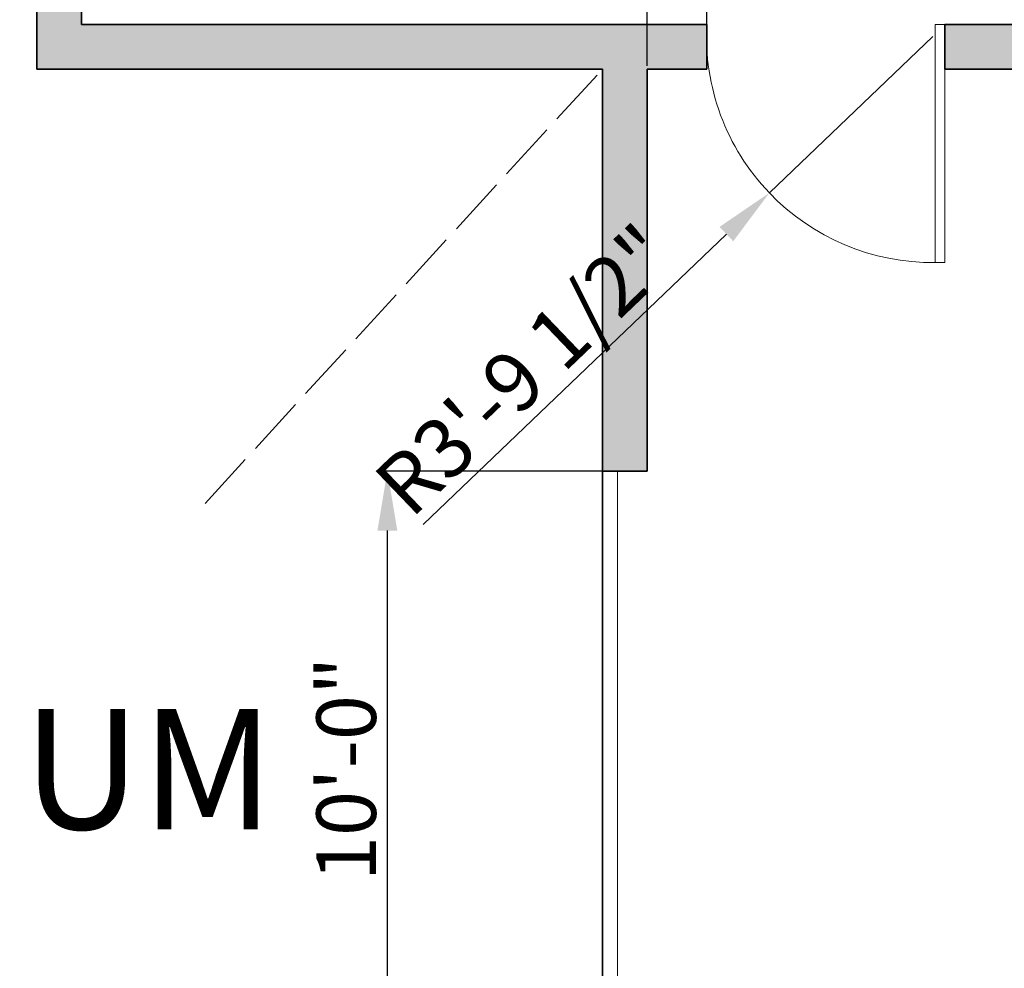
# Model space of a CAD drawing. Units: inches. Extents: x 2083 to 3317, y 1141 to 2115.
# Tile 116 of 256: x 2746 to 2944, y 1522 to 1713. Entities that reach past the tile are written whole.
import ezdxf

# ---------------------------------------------------------------- set-up
doc = ezdxf.new("R2010")
doc.units = ezdxf.units.IN
doc.linetypes.add('ACAD_ISO02W100', pattern=[15, 12, -3])
for name, color, linetype, lineweight in [('A-ANNO-DIMS', 2, 'Continuous', 18), ('A-AREA-IDEN', 7, 'Continuous', 25), ('A-DOOR', 4, 'Continuous', 18), ('A-FLOR-OPEN', 8, 'ACAD_ISO02W100', 13), ('A-GLAZ', 4, 'Continuous', 18), ('A-WALL', 7, 'Continuous', 35)]:
    doc.layers.add(name, color=color, linetype=linetype, lineweight=lineweight)
doc.layers.add('A-WALL-PATT', color=251, linetype='Continuous', lineweight=13, true_color=0x636466)
doc.styles.get("Standard").update_dxf_attribs({"font": 'arial.ttf'})
doc.dimstyles.new('ISO-25', dxfattribs={"dimtxt": 12, "dimasz": 12, "dimexe": 1.25, "dimexo": 0.625, "dimtad": 1, "dimlunit": 3, "dimtxsty": 'Standard', "dimcen": 2.5, "dimadec": 0, "dimazin": 0, "dimtfac": 1, "dimtmove": 0, "dimatfit": 3, "dimfxl": 1, "dimarcsym": 0})

# ---------------------------------------------------------------- blocks, each defined once
blk = doc.blocks.new('*D57')
at = {"layer": 'A-ANNO-DIMS', "color": 0, "lineweight": -2, "transparency": 16777216}
for p, q in [((2871.33, 1621.76), (2818.36, 1621.76)), ((2819.61, 1513.76), (2819.61, 1609.76)), ((2871.33, 1501.76), (2818.36, 1501.76))]:
    blk.add_line(p, q, dxfattribs=at)
at = {"layer": 'A-ANNO-DIMS', "color": 0, "transparency": 16777216}
for points in [[(2817.61, 1609.76), (2821.61, 1609.76), (2819.61, 1621.76)], [(2817.61, 1513.76), (2821.61, 1513.76), (2819.61, 1501.76)]]:
    blk.add_solid(points, dxfattribs=at)
at = {"layer": 'Defpoints', "color": 0, "transparency": 16777216}
for p in [(2819.61, 1621.76), (2871.96, 1621.76), (2871.96, 1501.76)]:
    blk.add_point(p, dxfattribs=at)
at = {"layer": 'A-ANNO-DIMS', "color": 0, "transparency": 16777216, "insert": (2812.86, 1561.76), "char_height": 12, "attachment_point": 5, "rotation": 90}
blk.add_mtext('10\'-0"', dxfattribs=at)
blk = doc.blocks.new('*D58')
at = {"layer": 'A-ANNO-DIMS', "color": 0, "lineweight": -2, "transparency": 16777216}
for p, q in [((2871.96, 1703.39), (2871.96, 1756.36)), ((2883.96, 1703.39), (2883.96, 1756.36)), ((2859.96, 1755.11), (2847.96, 1755.11)), ((2871.96, 1755.11), (2883.96, 1755.11)), ((2895.96, 1755.11), (2939.98, 1755.11))]:
    blk.add_line(p, q, dxfattribs=at)
at = {"layer": 'A-ANNO-DIMS', "color": 0, "transparency": 16777216}
for points in [[(2859.96, 1757.11), (2859.96, 1753.11), (2871.96, 1755.11)], [(2895.96, 1757.11), (2895.96, 1753.11), (2883.96, 1755.11)]]:
    blk.add_solid(points, dxfattribs=at)
at = {"layer": 'Defpoints', "color": 0, "transparency": 16777216}
for p in [(2883.96, 1755.11), (2871.96, 1702.76), (2883.96, 1702.76)]:
    blk.add_point(p, dxfattribs=at)
at = {"layer": 'A-ANNO-DIMS', "color": 0, "transparency": 16777216, "insert": (2923.97, 1761.86), "char_height": 12, "attachment_point": 5}
blk.add_mtext('1\'-0"', dxfattribs=at)
blk = doc.blocks.new('*D72')
at = {"layer": 'A-ANNO-DIMS', "color": 0, "lineweight": -2, "transparency": 16777216}
for p, q in [((2929.49, 1709.35), (2896.57, 1677.81)), ((2826.83, 1610.97), (2887.91, 1669.5))]:
    blk.add_line(p, q, dxfattribs=at)
at = {"layer": 'A-ANNO-DIMS', "color": 0, "transparency": 16777216}
blk.add_solid([(2886.52, 1670.95), (2889.29, 1668.06), (2896.57, 1677.81)], dxfattribs=at)
at = {"layer": 'Defpoints', "color": 0, "transparency": 16777216}
for p in [(2929.49, 1709.35), (2896.57, 1677.81)]:
    blk.add_point(p, dxfattribs=at)
at = {"layer": 'A-ANNO-DIMS', "color": 0, "transparency": 16777216, "insert": (2848.31, 1641.02), "char_height": 12, "attachment_point": 5, "rotation": 43.7815}
blk.add_mtext('R3\'-9 1/2"', dxfattribs=at)

msp = doc.modelspace()

# ---------------------------------------------------------------- hatches: boundary and pattern name
at = {"layer": 'A-WALL-PATT'}
h = msp.add_hatch(color=256, dxfattribs=at)
h.dxf.hatch_style = 1
h.paths.add_polyline_path([(3126.96, 2020.761), (2748.96, 2020.761), (2604.96, 2020.761), (2226.96, 2020.761), (2226.96, 1702.761), (2466.96, 1702.761), (2466.96, 1582.761), (2418.96, 1582.761), (2418.96, 1477.761), (2226.96, 1477.761), (2226.96, 1263.261), (2544.96, 1263.261), (2544.96, 1411.761), (2604.96, 1411.761), (2685.96, 1411.761), (2685.96, 1420.761), (2604.96, 1420.761), (2604.96, 1573.761), (2604.96, 1702.761), (2604.96, 2011.761), (2748.96, 2011.761), (2748.96, 1702.761), (2862.96, 1702.761), (2862.96, 1621.761), (2871.96, 1621.761), (2871.96, 1702.761), (2883.96, 1702.761), (2883.96, 1706.939, -0.0264593), (2883.96, 1711.761), (2757.96, 1711.761), (2757.96, 1807.761), (2787.96, 1807.761), (2787.96, 1812.261), (2757.96, 1812.261), (2757.96, 2011.761), (2877.96, 2011.761), (2877.96, 1812.261), (2847.96, 1812.261), (2847.96, 1807.761), (2889.836, 1807.761), (2889.836, 1812.261), (2882.46, 1812.261), (2882.46, 2011.761), (3117.96, 2011.761), (3117.96, 1812.261), (2937.836, 1812.261), (2937.836, 1807.761), (2995.71, 1807.761), (2995.71, 1796.118), (3000.21, 1796.118), (3000.21, 1807.761), (3117.96, 1807.761), (3117.96, 1711.761), (3000.21, 1711.761), (3000.21, 1760.118), (2998.573, 1760.118, -0.020711), (2995.71, 1760.118), (2995.71, 1711.761), (2931.96, 1711.761), (2931.96, 1702.761), (3126.96, 1702.761)])
h.paths.add_polyline_path([(2471.46, 2011.761), (2471.46, 1810.011), (2462.717, 1810.011), (2462.717, 1805.511), (2505.96, 1805.511), (2505.96, 1810.011), (2475.96, 1810.011), (2475.96, 2011.761), (2595.96, 2011.761), (2595.96, 1810.011), (2565.96, 1810.011), (2565.96, 1805.511), (2595.96, 1805.511), (2595.96, 1711.761), (2235.96, 1711.761), (2235.96, 1805.511), (2353.71, 1805.511), (2353.71, 1796.054), (2358.21, 1796.054), (2358.21, 1805.511), (2414.717, 1805.511), (2414.717, 1810.011), (2235.96, 1810.011), (2235.96, 2011.761)], flags=16)
h.paths.add_polyline_path([(2270.205, 1994.61), (2270.205, 1970.61), (2246.205, 1970.61), (2246.205, 1994.61)], flags=0)
edge = h.paths.add_edge_path(flags=0)
edge.add_ellipse((2332.027, 1899.798), major_axis=(-3.043, 3.043), ratio=0.1682525, start_angle=-161.33217, end_angle=-156.30711, ccw=False)
edge.add_ellipse((2333.082, 1898.744), major_axis=(-1.055, 1.055), ratio=0.4535321, start_angle=-123.37102, end_angle=-94.15911)
edge = h.paths.add_edge_path(flags=0)
edge.add_ellipse((2332.027, 1968.876), major_axis=(3.043, 3.043), ratio=0.1682525, start_angle=18.66783, end_angle=23.69289)
edge.add_spline(control_points=[(2332.926, 1970.691), (2332.227, 1970.336), (2330.894, 1969.659), (2328.413, 1970.932), (2327.204, 1967.749), (2324.71, 1969.956), (2322.533, 1967.012), (2320.013, 1971.296), (2317.68, 1968.158), (2316.041, 1967.102), (2315.427, 1966.81)], knot_values=[0, 0, 0, 0, 2.2670587, 4.3245589, 6.6855835, 8.8786411, 11.121502, 14.300359, 17.7552837, 19.732645, 19.732645, 19.732645, 19.732645], degree=3, periodic=0)
edge.add_ellipse((2332.027, 1968.876), major_axis=(3.043, 3.043), ratio=0.1682525, start_angle=18.66783, end_angle=23.69289, ccw=False)
edge.add_ellipse((2333.082, 1969.931), major_axis=(1.055, 1.055), ratio=0.4535321, start_angle=56.62898, end_angle=85.84089, ccw=False)
edge = h.paths.add_edge_path(flags=0)
edge.add_spline(control_points=[(2296.428, 1967.988), (2293.628, 1965.336), (2287.704, 1959.727), (2299.744, 1949.996), (2294.533, 1935.669), (2290.573, 1920.604), (2293.394, 1909.974), (2296.185, 1904.967)], knot_values=[0.0991853, 0.0991853, 0.0991853, 0.0991853, 0.3453009, 0.6198217, 0.9826526, 1.3860932, 1.8105546, 1.8105546, 1.8105546, 1.8105546], degree=3, periodic=0)
edge.add_spline(control_points=[(2296.185, 1904.967), (2297.384, 1902.619), (2298.001, 1901.949), (2298.553, 1901.468)], knot_values=[0.0062457, 0.0062457, 0.0062457, 0.0062457, 0.0554759, 0.0554759, 0.0554759, 0.0554759], degree=3, periodic=0)
edge.add_spline(control_points=[(2298.553, 1901.468), (2297.259, 1900.923), (2295.225, 1900.232), (2293.06, 1900.614), (2292.101, 1900.788), (2292.09, 1900.791)], knot_values=[0.3128349, 0.3128349, 0.3128349, 0.3128349, 0.4017797, 0.4749867, 0.4759027, 0.4759027, 0.4759027, 0.4759027], degree=3, periodic=0)
edge.add_arc((2292.794, 1904.664), 3.937, 215.4209, 259.69818, ccw=False)
edge.add_spline(control_points=[(2289.585, 1902.382), (2289.477, 1902.535), (2289.368, 1902.688), (2289.261, 1902.841)], knot_values=[0.1028719, 0.1028719, 0.1028719, 0.1028719, 0.1168958, 0.1168958, 0.1168958, 0.1168958], degree=3, periodic=0)
edge.add_spline(control_points=[(2289.261, 1902.841), (2288.687, 1902.55), (2287.64, 1902.02), (2285.881, 1901.874), (2283.853, 1901.504), (2281.72, 1899.711), (2278.467, 1899.493), (2276.157, 1901.883), (2272.259, 1899.804), (2267.778, 1901.843), (2262.244, 1900.184), (2257.415, 1901.782), (2254.318, 1900.726), (2253.178, 1900.337)], knot_values=[0, 0, 0, 0, 1.9079767, 3.4771759, 5.261074, 7.9728515, 11.6802485, 13.7179214, 16.9395917, 22.789562, 27.5025027, 33.5952153, 37.1456181, 37.1456181, 37.1456181, 37.1456181], degree=3, periodic=0)
edge.add_line((2253.178, 1900.337), (2250.244, 1902.841))
edge.add_line((2250.244, 1902.841), (2250.244, 1965.833))
edge.add_line((2250.244, 1965.833), (2253.178, 1968.337))
edge.add_spline(control_points=[(2253.178, 1968.337), (2254.318, 1967.948), (2257.415, 1966.892), (2262.244, 1968.49), (2267.778, 1966.831), (2271.527, 1968.537), (2273.876, 1967.828), (2274.207, 1967.728)], knot_values=[0, 0, 0, 0, 0.0901802, 0.2449351, 0.3646438, 0.5132331, 0.5378548, 0.5378548, 0.5378548, 0.5378548], degree=3, periodic=0)
edge.add_arc((2274.353, 1963.793), 3.937, 72.05113, 92.12795, ccw=False)
edge.add_arc((2281.297, 1985.23), 18.596, 252.05113, 288.56572)
edge.add_arc((2292.317, 1956.029), 12.646, 71.02679, 113.77822, ccw=False)
edge = h.paths.add_edge_path(flags=0)
edge.add_spline(control_points=[(2274.899, 1951.856), (2275.066, 1951.617), (2275.233, 1951.377), (2275.398, 1951.136)], knot_values=[1.4099157, 1.4099157, 1.4099157, 1.4099157, 1.4315903, 1.4315903, 1.4315903, 1.4315903], degree=3, periodic=0)
edge.add_spline(control_points=[(2275.398, 1951.136), (2275.792, 1950.562), (2276.179, 1949.984), (2276.546, 1949.397)], knot_values=[1.3582378, 1.3582378, 1.3582378, 1.3582378, 1.4099157, 1.4099157, 1.4099157, 1.4099157], degree=3, periodic=0)
edge.add_line((2276.546, 1949.397), (2277.437, 1947.862))
edge.add_spline(control_points=[(2277.437, 1947.862), (2276.304, 1945.673), (2274.64, 1942.427), (2274.632, 1938.094), (2272.799, 1930.852), (2274.356, 1943.897), (2275.948, 1947.923), (2276.546, 1949.397)], knot_values=[0.0056315, 0.0056315, 0.0056315, 0.0056315, 0.1860139, 0.2660015, 0.3570872, 0.5963902, 0.7397317, 0.7397317, 0.7397317, 0.7397317], degree=3, periodic=0)
edge.add_spline(control_points=[(2276.546, 1949.397), (2276.179, 1949.984), (2275.792, 1950.562), (2275.398, 1951.136)], knot_values=[1.3582378, 1.3582378, 1.3582378, 1.3582378, 1.4099157, 1.4099157, 1.4099157, 1.4099157], degree=3, periodic=0)
edge.add_spline(control_points=[(2275.398, 1951.136), (2274.943, 1950.08), (2274.208, 1948.025), (2273.935, 1944.851), (2272.469, 1937.627), (2273.466, 1945.696), (2274.701, 1951.059), (2274.899, 1951.856)], knot_values=[0.1043639, 0.1043639, 0.1043639, 0.1043639, 0.1896363, 0.2696239, 0.3607096, 0.6000126, 0.6446217, 0.6446217, 0.6446217, 0.6446217], degree=3, periodic=0)
h.paths.add_polyline_path([(2269.168, 1963.128, -0.3575267), (2268.171, 1960.976, -0.0925607), (2268.171, 1939.436, -0.3575267), (2269.168, 1937.285, -0.3575267), (2267.016, 1938.282, -0.1647847), (2254.686, 1938.282, -0.3575267), (2252.534, 1937.285, -0.3575267), (2253.531, 1939.436, -0.0925607), (2253.531, 1960.976, -0.3575267), (2252.534, 1963.128, -0.3575267), (2254.686, 1962.131, -0.1647847), (2267.016, 1962.131, -0.3575267)], flags=0)
h.paths.add_polyline_path([(2248.874, 1967.802), (2248.874, 1957.028), (2249.458, 1957.028), (2249.458, 1911.647), (2248.874, 1911.647), (2248.874, 1900.873), (2246.512, 1900.873, 0.1973271), (2244.15, 1902.457), (2244.15, 1966.218, 0.1973271), (2246.512, 1967.802)], flags=0)
h.paths.add_polyline_path([(2269.168, 1931.389, -0.3575267), (2268.171, 1929.238, -0.0925607), (2268.171, 1907.698, -0.3575267), (2269.168, 1905.547, -0.3575267), (2267.016, 1906.544, -0.1647847), (2254.686, 1906.544, -0.3575267), (2252.534, 1905.547, -0.3575267), (2253.531, 1907.698, -0.0925607), (2253.531, 1929.238, -0.3575267), (2252.534, 1931.389, -0.3575267), (2254.686, 1930.392, -0.1647847), (2267.016, 1930.392, -0.3575267)], flags=0)
edge = h.paths.add_edge_path(flags=0)
edge.add_spline(control_points=[(2276.197, 1906.724), (2276.168, 1909.029), (2276.114, 1913.372), (2270.598, 1924.925), (2273.905, 1919.013), (2275.922, 1916.262), (2275.475, 1912.402), (2277.258, 1910.381), (2276.696, 1908.225), (2276.646, 1906.813), (2276.618, 1906.008)], knot_values=[0, 0, 0, 0, 8.6102597, 16.2212739, 18.8430575, 23.8048978, 27.4408283, 29.3561016, 31.2034776, 33.6506866, 33.6506866, 33.6506866, 33.6506866], degree=3, periodic=0)
edge.add_spline(control_points=[(2276.618, 1906.008), (2276.623, 1905.624), (2276.498, 1904.629), (2275.442, 1903.855), (2274.937, 1903.08), (2274.859, 1902.841)], knot_values=[0.1564884, 0.1564884, 0.1564884, 0.1564884, 0.1843975, 0.2313765, 0.2505985, 0.2505985, 0.2505985, 0.2505985], degree=3, periodic=0)
edge.add_line((2274.859, 1902.841), (2276.506, 1902.841))
edge.add_spline(control_points=[(2276.506, 1902.841), (2276.788, 1903.085), (2277.665, 1904.125), (2278.25, 1904.341), (2277.654, 1908.527), (2278.156, 1906.228), (2278.1, 1905.286), (2278.847, 1904.069), (2277.857, 1903.415), (2277.874, 1902.991), (2277.904, 1902.841)], knot_values=[0.0595743, 0.0595743, 0.0595743, 0.0595743, 0.0807529, 0.1037415, 0.1697201, 0.1760361, 0.2071372, 0.2404744, 0.2623409, 0.2736605, 0.2736605, 0.2736605, 0.2736605], degree=3, periodic=0)
edge.add_line((2277.904, 1902.841), (2280.03, 1902.841))
edge.add_spline(control_points=[(2280.03, 1902.841), (2279.888, 1903.088), (2279.499, 1903.982), (2280.152, 1905.939), (2278.104, 1909.658), (2279.762, 1907.185), (2280.328, 1904.875), (2280.485, 1903.49), (2281.463, 1903.249), (2281.758, 1902.936), (2281.834, 1902.841)], knot_values=[0.013856, 0.013856, 0.013856, 0.013856, 0.0348738, 0.0888667, 0.1078792, 0.1267378, 0.158714, 0.1937575, 0.2174868, 0.2267221, 0.2267221, 0.2267221, 0.2267221], degree=3, periodic=0)
edge.add_spline(control_points=[(2281.834, 1902.841), (2281.788, 1902.827), (2281.647, 1902.783), (2281.396, 1902.859), (2281.088, 1902.985), (2280.721, 1903.061), (2280.333, 1903.026), (2280.125, 1902.899), (2280.03, 1902.841)], knot_values=[0, 0, 0, 0, 0.1441304, 0.435517, 0.7492759, 1.1530457, 1.5483707, 1.878348, 1.878348, 1.878348, 1.878348], degree=3, periodic=0)
edge.add_line((2280.03, 1902.841), (2277.904, 1902.841))
edge.add_spline(control_points=[(2277.904, 1902.841), (2277.893, 1902.796), (2277.865, 1902.68), (2277.607, 1902.687), (2277.274, 1902.801), (2276.838, 1902.62), (2276.584, 1902.789), (2276.506, 1902.841)], knot_values=[0, 0, 0, 0, 0.1271885, 0.3261988, 0.6280094, 1.2435704, 1.5153306, 1.5153306, 1.5153306, 1.5153306], degree=3, periodic=0)
edge.add_line((2276.506, 1902.841), (2274.859, 1902.841))
edge.add_spline(control_points=[(2274.859, 1902.841), (2274.814, 1902.899), (2274.725, 1903.013), (2274.493, 1903.119), (2274.244, 1902.961), (2273.937, 1903.185), (2273.614, 1902.983), (2273.408, 1902.883), (2273.322, 1902.841)], knot_values=[0, 0, 0, 0, 0.2184302, 0.4369566, 0.6879766, 0.9903786, 1.3983955, 1.6918498, 1.6918498, 1.6918498, 1.6918498], degree=3, periodic=0)
edge.add_spline(control_points=[(2273.322, 1902.841), (2273.617, 1903.446), (2274.274, 1904.538), (2276.027, 1904.574), (2276.207, 1906.584), (2276.197, 1906.724)], knot_values=[0.0122268, 0.0122268, 0.0122268, 0.0122268, 0.0594721, 0.1062177, 0.134458, 0.134458, 0.134458, 0.134458], degree=3, periodic=0)
h.paths.add_polyline_path([(2270.776, 1897.79), (2270.776, 1873.79), (2246.776, 1873.79), (2246.776, 1897.79)], flags=0)
h.paths.add_polyline_path([(2353.71, 1760.005), (2353.71, 1760.054), (2358.21, 1760.054, -0.033729)], flags=0)
h.paths.add_polyline_path([(2321.819, 1737.529), (2341.995, 1737.529, -0.4142136), (2343.203, 1736.321), (2343.203, 1721.021, -0.4142136), (2341.995, 1719.813), (2321.819, 1719.813, -0.4142136), (2320.611, 1721.021), (2320.611, 1736.321, -0.4142136)], flags=0)
h.paths.add_polyline_path([(2324.235, 1736.321), (2339.579, 1736.321, -0.4142136), (2341.995, 1733.905), (2341.995, 1725.45, -0.4142136), (2339.579, 1723.034), (2333.681, 1723.034), (2333.845, 1722.045, -0.8706461), (2335.425, 1721.826, -0.767327), (2333.923, 1721.423), (2331.291, 1721.423, -0.767327), (2329.788, 1721.826, -0.8706461), (2331.368, 1722.045), (2331.533, 1723.034), (2324.235, 1723.034, -0.4142136), (2321.819, 1725.45), (2321.819, 1733.905, -0.4142136)], flags=0)
h.paths.add_polyline_path([(2570.484, 1928.615), (2589.684, 1928.615), (2590.169, 1928.615), (2590.169, 1904.993), (2570.484, 1904.993)], flags=0)
h.paths.add_polyline_path([(2574.447, 1927.264, -1), (2572.829, 1927.264, -1)], flags=0)
h.paths.add_polyline_path([(2573.09, 1926.941), (2573.925, 1927.776), (2574.148, 1927.553), (2573.313, 1926.718)], flags=0)
h.paths.add_polyline_path([(2578.779, 1919.73, -1), (2571.592, 1919.73, -1)], flags=0)
h.paths.add_polyline_path([(2578.385, 1919.73, -1), (2571.985, 1919.73, -1)], flags=0)
h.paths.add_polyline_path([(2331.596, 1729.476, -1), (2333.618, 1729.476, -1)], flags=0)
h.paths.add_polyline_path([(2578.034, 1927.264, -1), (2576.416, 1927.264, -1)], flags=0)
h.paths.add_polyline_path([(2576.689, 1927.531), (2576.912, 1927.754), (2577.747, 1926.919), (2577.524, 1926.696)], flags=0)
h.paths.add_polyline_path([(2578.139, 1909.86, -1), (2572.232, 1909.86, -1)], flags=0)
h.paths.add_polyline_path([(2577.745, 1909.86, -1), (2572.625, 1909.86, -1)], flags=0)
h.paths.add_polyline_path([(2583.798, 1927.264, -1), (2582.179, 1927.264, -1)], flags=0)
h.paths.add_polyline_path([(2582.719, 1927.754), (2583.554, 1926.919), (2583.331, 1926.696), (2582.496, 1927.531)], flags=0)
h.paths.add_polyline_path([(2582.496, 1927.531), (2582.719, 1927.754), (2583.554, 1926.919), (2583.331, 1926.696)], flags=0)
h.paths.add_polyline_path([(2587.739, 1920.53, -1), (2581.832, 1920.53, -1)], flags=0)
h.paths.add_polyline_path([(2587.345, 1920.53, -1), (2582.225, 1920.53, -1)], flags=0)
h.paths.add_polyline_path([(2587.385, 1927.264, -1), (2585.766, 1927.264, -1)], flags=0)
h.paths.add_polyline_path([(2586.082, 1926.98), (2586.917, 1927.815), (2587.14, 1927.593), (2586.305, 1926.758)], flags=0)
h.paths.add_polyline_path([(2588.379, 1910.66, -1), (2581.192, 1910.66, -1)], flags=0)
h.paths.add_polyline_path([(2587.985, 1910.66, -1), (2581.585, 1910.66, -1)], flags=0)
h.paths.add_polyline_path([(2417.168, 1729.478), (2437.344, 1729.478, -0.4142136), (2438.552, 1728.27), (2438.552, 1712.969, -0.4142136), (2437.344, 1711.761), (2417.168, 1711.761, -0.4142136), (2415.96, 1712.969), (2415.96, 1728.27, -0.4142136)], flags=0)
h.paths.add_polyline_path([(2419.584, 1728.27), (2434.928, 1728.27, -0.4142136), (2437.344, 1725.854), (2437.344, 1717.398, -0.4142136), (2434.928, 1714.983), (2429.029, 1714.983), (2429.194, 1713.994, -0.8706461), (2430.774, 1713.775, -0.767327), (2429.271, 1713.372), (2426.64, 1713.372, -0.767327), (2425.137, 1713.775, -0.8706461), (2426.717, 1713.994), (2426.882, 1714.983), (2419.584, 1714.983, -0.4142136), (2417.168, 1717.398), (2417.168, 1725.854, -0.4142136)], flags=0)
h.paths.add_polyline_path([(2419.584, 1728.27), (2434.928, 1728.27, -0.4142136), (2437.344, 1725.854), (2437.344, 1717.398, -0.4142136), (2434.928, 1714.983), (2429.029, 1714.983), (2428.358, 1719.009), (2427.553, 1719.009), (2426.882, 1714.983), (2419.584, 1714.983, -0.4142136), (2417.168, 1717.398), (2417.168, 1725.854, -0.4142136)], flags=0)
h.paths.add_polyline_path([(2426.944, 1721.425, -1), (2428.967, 1721.425, -1)], flags=0)
h.paths.add_polyline_path([(2475.96, 1702.761), (2595.96, 1702.761), (2595.96, 1582.761), (2475.96, 1582.761)], flags=16)
h.paths.add_polyline_path([(2427.96, 1573.761), (2595.96, 1573.761), (2595.96, 1468.761), (2595.96, 1420.761), (2384.46, 1420.761), (2384.46, 1468.761), (2427.96, 1468.761)], flags=16)
h.paths.add_polyline_path([(2379.96, 1468.761), (2379.96, 1420.761), (2235.96, 1420.761), (2235.96, 1468.761)], flags=16)
h.paths.add_polyline_path([(2317.816, 1466.696), (2337.992, 1466.696, -0.4142136), (2339.2, 1465.488), (2339.2, 1450.187, -0.4142136), (2337.992, 1448.979), (2317.816, 1448.979, -0.4142136), (2316.608, 1450.187), (2316.608, 1465.488, -0.4142136)], flags=0)
h.paths.add_polyline_path([(2320.232, 1465.488), (2335.576, 1465.488, -0.4142136), (2337.992, 1463.072), (2337.992, 1454.616, -0.4142136), (2335.576, 1452.2), (2329.677, 1452.2), (2329.842, 1451.212, -0.8706461), (2331.422, 1450.992, -0.767327), (2329.92, 1450.59), (2327.288, 1450.59, -0.767327), (2325.785, 1450.992, -0.8706461), (2327.365, 1451.212), (2327.53, 1452.2), (2320.232, 1452.2, -0.4142136), (2317.816, 1454.616), (2317.816, 1463.072, -0.4142136)], flags=0)
h.paths.add_polyline_path([(2320.232, 1465.488), (2335.576, 1465.488, -0.4142136), (2337.992, 1463.072), (2337.992, 1454.616, -0.4142136), (2335.576, 1452.2), (2329.677, 1452.2), (2329.006, 1456.227), (2328.201, 1456.227), (2327.53, 1452.2), (2320.232, 1452.2, -0.4142136), (2317.816, 1454.616), (2317.816, 1463.072, -0.4142136)], flags=0)
h.paths.add_polyline_path([(2327.593, 1458.643, -1), (2329.615, 1458.643, -1)], flags=0)
h.paths.add_polyline_path([(2244.412, 1433.34), (2241.921, 1433.34, -0.4142136), (2240.018, 1435.244), (2240.018, 1440.953, -0.4142105), (2241.921, 1442.856), (2244.412, 1442.856, -1.9764724)], flags=0)
h.paths.add_polyline_path([(2245.357, 1434.398, -0.4142136), (2245.357, 1441.799, -2.1440985)], flags=0)
h.paths.add_polyline_path([(2535.96, 1416.261), (2535.96, 1272.261), (2235.96, 1272.261), (2235.96, 1416.261)], flags=16)
h.paths.add_polyline_path([(2260.12, 1384.293), (2260.12, 1362.039), (2237.865, 1362.039), (2237.865, 1384.293)], flags=0)
edge = h.paths.add_edge_path(flags=0)
edge.add_line((2318.252, 1362.093), (2318.146, 1362.001))
edge.add_ellipse((2317.445, 1360.431), major_axis=(2.822, 2.822), ratio=0.1682525, start_angle=18.66783, end_angle=20.94813, ccw=False)
edge.add_ellipse((2318.423, 1361.409), major_axis=(0.978, 0.978), ratio=0.4535321, start_angle=56.62898, end_angle=70.2262, ccw=False)
edge = h.paths.add_edge_path(flags=0)
edge.add_line((2319.107, 1295.571), (2319.015, 1295.677))
edge.add_ellipse((2317.445, 1296.378), major_axis=(-2.822, 2.822), ratio=0.1682525, start_angle=-161.33217, end_angle=-159.05187, ccw=False)
edge.add_ellipse((2318.423, 1295.4), major_axis=(-0.978, 0.978), ratio=0.4535321, start_angle=-123.37102, end_angle=-109.7738)
edge = h.paths.add_edge_path(flags=0)
edge.add_spline(control_points=[(2284.21, 1301.17), (2284.581, 1300.445), (2284.891, 1299.892), (2285.16, 1299.461)], knot_values=[0.0390658, 0.0390658, 0.0390658, 0.0390658, 0.0554759, 0.0554759, 0.0554759, 0.0554759], degree=3, periodic=0)
edge.add_line((2285.16, 1299.461), (2284.21, 1301.17))
edge = h.paths.add_edge_path(flags=0)
edge.add_line((2280.412, 1297.298), (2283.37, 1297.036))
edge.add_line((2283.37, 1297.036), (2286.406, 1297.926))
edge.add_spline(control_points=[(2286.406, 1297.926), (2285.305, 1297.463), (2284.345, 1297.129), (2283.37, 1297.036)], knot_values=[0.3943688, 0.3943688, 0.3943688, 0.3943688, 0.4759027, 0.4759027, 0.4759027, 0.4759027], degree=3, periodic=0)
edge.add_spline(control_points=[(2283.37, 1297.036), (2283.281, 1297.028), (2282.316, 1296.957), (2281.313, 1297.134), (2280.423, 1297.296), (2280.412, 1297.298)], knot_values=[0.3128349, 0.3128349, 0.3128349, 0.3128349, 0.3202458, 0.3934528, 0.3943688, 0.3943688, 0.3943688, 0.3943688], degree=3, periodic=0)
edge = h.paths.add_edge_path(flags=0)
edge.add_line((2284.436, 1359.607), (2280.446, 1355.328))
edge.add_line((2280.446, 1355.328), (2279.58, 1351.018))
edge.add_line((2279.58, 1351.018), (2282.413, 1346.58))
edge.add_spline(control_points=[(2282.413, 1346.58), (2283.153, 1345.589), (2284.253, 1344.029), (2284.801, 1342.387), (2284.935, 1341.806)], knot_values=[1.2400982, 1.2400982, 1.2400982, 1.2400982, 1.3328922, 1.3827123, 1.3827123, 1.3827123, 1.3827123], degree=3, periodic=0)
edge.add_spline(control_points=[(2284.935, 1341.806), (2285.319, 1340.141), (2285.233, 1338.409), (2284.91, 1336.654)], knot_values=[1.0974841, 1.0974841, 1.0974841, 1.0974841, 1.2400982, 1.2400982, 1.2400982, 1.2400982], degree=3, periodic=0)
edge.add_spline(control_points=[(2284.91, 1336.654), (2284.587, 1334.899), (2284.027, 1333.12), (2283.463, 1331.361)], knot_values=[0.9548699, 0.9548699, 0.9548699, 0.9548699, 1.0974841, 1.0974841, 1.0974841, 1.0974841], degree=3, periodic=0)
edge.add_line((2283.463, 1331.361), (2281.89, 1326.153))
edge.add_line((2281.89, 1326.153), (2280.756, 1321.056))
edge.add_line((2280.756, 1321.056), (2280.299, 1316.002))
edge.add_line((2280.299, 1316.002), (2280.716, 1310.95))
edge.add_line((2280.716, 1310.95), (2282.028, 1305.972))
edge.add_line((2282.028, 1305.972), (2284.21, 1301.17))
edge.add_spline(control_points=[(2284.21, 1301.17), (2283.341, 1302.73), (2282.612, 1304.336), (2282.028, 1305.972)], knot_values=[0.0991853, 0.0991853, 0.0991853, 0.0991853, 0.2417994, 0.2417994, 0.2417994, 0.2417994], degree=3, periodic=0)
edge.add_spline(control_points=[(2282.028, 1305.972), (2281.444, 1307.608), (2281.005, 1309.273), (2280.716, 1310.95)], knot_values=[0.2417994, 0.2417994, 0.2417994, 0.2417994, 0.3844135, 0.3844135, 0.3844135, 0.3844135], degree=3, periodic=0)
edge.add_spline(control_points=[(2280.716, 1310.95), (2280.433, 1312.588), (2280.289, 1314.277), (2280.299, 1315.962), (2280.299, 1316.002)], knot_values=[0.3844135, 0.3844135, 0.3844135, 0.3844135, 0.5236467, 0.5270276, 0.5270276, 0.5270276, 0.5270276], degree=3, periodic=0)
edge.add_spline(control_points=[(2280.299, 1316.002), (2280.312, 1317.687), (2280.478, 1319.368), (2280.756, 1321.056)], knot_values=[0.5270276, 0.5270276, 0.5270276, 0.5270276, 0.6696417, 0.6696417, 0.6696417, 0.6696417], degree=3, periodic=0)
edge.add_spline(control_points=[(2280.756, 1321.056), (2281.035, 1322.744), (2281.426, 1324.44), (2281.89, 1326.153)], knot_values=[0.6696417, 0.6696417, 0.6696417, 0.6696417, 0.8122558, 0.8122558, 0.8122558, 0.8122558], degree=3, periodic=0)
edge.add_spline(control_points=[(2281.89, 1326.153), (2282.264, 1327.533), (2282.788, 1329.262), (2283.353, 1331.018), (2283.463, 1331.361)], knot_values=[0.8122558, 0.8122558, 0.8122558, 0.8122558, 0.9270873, 0.9548699, 0.9548699, 0.9548699, 0.9548699], degree=3, periodic=0)
edge.add_line((2283.463, 1331.361), (2284.91, 1336.654))
edge.add_line((2284.91, 1336.654), (2284.935, 1341.806))
edge.add_line((2284.935, 1341.806), (2282.413, 1346.58))
edge.add_spline(control_points=[(2282.413, 1346.58), (2281.275, 1348.104), (2280.078, 1349.57), (2279.58, 1351.018)], knot_values=[1.3827123, 1.3827123, 1.3827123, 1.3827123, 1.5253264, 1.5253264, 1.5253264, 1.5253264], degree=3, periodic=0)
edge.add_spline(control_points=[(2279.58, 1351.018), (2279.443, 1351.415), (2279.136, 1352.857), (2279.735, 1354.29), (2280.446, 1355.328)], knot_values=[1.5253264, 1.5253264, 1.5253264, 1.5253264, 1.564439, 1.6679405, 1.6679405, 1.6679405, 1.6679405], degree=3, periodic=0)
edge.add_spline(control_points=[(2280.446, 1355.328), (2281.426, 1356.758), (2282.931, 1358.183), (2284.436, 1359.607)], knot_values=[1.6679405, 1.6679405, 1.6679405, 1.6679405, 1.8105546, 1.8105546, 1.8105546, 1.8105546], degree=3, periodic=0)
edge.add_arc((2280.623, 1348.518), 11.726, 71.02679, 113.77822)
edge.add_arc((2270.405, 1375.595), 17.244, 252.05113, 288.56572, ccw=False)
edge.add_arc((2263.966, 1355.718), 3.651, 72.05113, 92.12795)
edge.add_arc((2263.966, 1355.718), 3.651, 92.12795, 177.98513)
edge.add_spline(control_points=[(2260.318, 1355.846), (2260.26, 1354.221), (2260.551, 1350.187), (2262.999, 1346.766), (2264.473, 1344.649)], knot_values=[1.4315903, 1.4315903, 1.4315903, 1.4315903, 1.5641438, 1.7706953, 1.7706953, 1.7706953, 1.7706953], degree=3, periodic=0)
edge.add_line((2264.473, 1344.649), (2264.936, 1343.983))
edge.add_spline(control_points=[(2263.801, 1340.248), (2263.843, 1340.514), (2264.067, 1341.756), (2264.513, 1343.002), (2264.935, 1343.981)], knot_values=[0.5365702, 0.5365702, 0.5365702, 0.5365702, 0.5593494, 0.6446217, 0.6446217, 0.6446217, 0.6446217], degree=3, periodic=0)
edge.add_spline(control_points=[(2264.935, 1343.981), (2265.118, 1343.715), (2265.299, 1343.448), (2265.477, 1343.179)], knot_values=[1.3840767, 1.3840767, 1.3840767, 1.3840767, 1.4099157, 1.4099157, 1.4099157, 1.4099157], degree=3, periodic=0)
edge.add_spline(control_points=[(2265.477, 1343.179), (2265.655, 1342.911), (2265.829, 1342.641), (2265.999, 1342.369)], knot_values=[1.3582378, 1.3582378, 1.3582378, 1.3582378, 1.3840767, 1.3840767, 1.3840767, 1.3840767], degree=3, periodic=0)
edge.add_line((2265.999, 1342.369), (2266.826, 1340.946))
edge.add_spline(control_points=[(2266.826, 1340.946), (2268.894, 1337.09), (2271.398, 1325.843), (2270.516, 1310.569), (2275.919, 1301.861), (2277.79, 1299.199)], knot_values=[0.1168958, 0.1168958, 0.1168958, 0.1168958, 0.4729873, 1.0509689, 1.3137934, 1.3137934, 1.3137934, 1.3137934], degree=3, periodic=0)
edge.add_spline(control_points=[(2277.79, 1299.199), (2277.839, 1299.128), (2277.889, 1299.057), (2277.94, 1298.987)], knot_values=[0.1098839, 0.1098839, 0.1098839, 0.1098839, 0.1168958, 0.1168958, 0.1168958, 0.1168958], degree=3, periodic=0)
edge.add_line((2277.94, 1298.987), (2277.789, 1299.199))
edge.add_spline(control_points=[(2277.789, 1299.199), (2277.257, 1298.929), (2276.286, 1298.438), (2275.039, 1298.334), (2274.383, 1298.239), (2274.215, 1298.209)], knot_values=[33.1218702, 33.1218702, 33.1218702, 33.1218702, 35.0290557, 36.5982549, 37.1448269, 37.1448269, 37.1448269, 37.1448269], degree=3, periodic=0)
edge.add_line((2274.215, 1298.209), (2273.073, 1297.893))
edge.add_spline(control_points=[(2273.073, 1297.893), (2272.323, 1297.58), (2271.039, 1296.511), (2269.248, 1296.226), (2268.423, 1296.375)], knot_values=[26.5325843, 26.5325843, 26.5325843, 26.5325843, 29.198919, 31.8391012, 31.8391012, 31.8391012, 31.8391012], degree=3, periodic=0)
edge.add_line((2268.423, 1296.375), (2263.879, 1297.458))
edge.add_spline(control_points=[(2263.879, 1297.458), (2263.556, 1297.359), (2261.86, 1296.839), (2260.239, 1297.282), (2258.933, 1297.516)], knot_values=[15.9195506, 15.9195506, 15.9195506, 15.9195506, 16.9395917, 21.2260675, 21.2260675, 21.2260675, 21.2260675], degree=3, periodic=0)
edge.add_line((2258.933, 1297.516), (2254.055, 1297.329))
edge.add_spline(control_points=[(2254.055, 1297.329), (2253.756, 1297.296), (2252.114, 1297.165), (2250.462, 1297.544), (2249.13, 1297.668)], knot_values=[5.3065169, 5.3065169, 5.3065169, 5.3065169, 6.2764352, 10.6130337, 10.6130337, 10.6130337, 10.6130337], degree=3, periodic=0)
edge.add_line((2249.13, 1297.668), (2244.332, 1296.878))
edge.add_line((2244.332, 1296.878), (2241.611, 1299.199))
edge.add_line((2241.611, 1299.199), (2241.611, 1357.609))
edge.add_line((2241.611, 1357.609), (2244.332, 1359.931))
edge.add_line((2244.332, 1359.931), (2252.729, 1359.543))
edge.add_spline(control_points=[(2252.729, 1359.543), (2252.871, 1359.546), (2253.306, 1359.548), (2253.74, 1359.514), (2254.032, 1359.482)], knot_values=[0.233291, 0.233291, 0.233291, 0.233291, 0.2449351, 0.2689274, 0.2689274, 0.2689274, 0.2689274], degree=3, periodic=0)
edge.add_line((2254.032, 1359.482), (2259.587, 1359.416))
edge.add_spline(control_points=[(2259.587, 1359.416), (2260.677, 1359.629), (2262.073, 1359.897), (2263.524, 1359.459), (2263.83, 1359.366)], knot_values=[0.4225164, 0.4225164, 0.4225164, 0.4225164, 0.5132331, 0.5378548, 0.5378548, 0.5378548, 0.5378548], degree=3, periodic=0)
edge.add_arc((2263.966, 1355.718), 3.651, 72.05113, 92.12795, ccw=False)
edge.add_arc((2270.405, 1375.595), 17.244, 252.05113, 288.56572)
edge.add_arc((2280.623, 1348.518), 11.726, 71.02679, 113.77822, ccw=False)
h.paths.add_polyline_path([(2240.341, 1359.435), (2240.341, 1349.444), (2240.882, 1349.444), (2240.882, 1307.365), (2240.341, 1307.365), (2240.341, 1297.374), (2238.15, 1297.374, 0.1973271), (2235.96, 1298.843), (2235.96, 1357.966, 0.1973271), (2238.15, 1359.435)], flags=0)
h.paths.add_polyline_path([(2259.158, 1355.101, -0.3575267), (2258.233, 1353.106, -0.0925607), (2258.233, 1333.133, -0.3575267), (2259.158, 1331.138, -0.3575267), (2257.163, 1332.062, -0.1647847), (2245.729, 1332.062, -0.3575267), (2243.735, 1331.138, -0.3575267), (2244.659, 1333.133, -0.0925607), (2244.659, 1353.106, -0.3575267), (2243.735, 1355.101, -0.3575267), (2245.729, 1354.176, -0.1647847), (2257.163, 1354.176, -0.3575267)], flags=0)
edge = h.paths.add_edge_path(flags=0)
edge.add_line((2265.999, 1342.369), (2266.826, 1340.946))
edge.add_line((2266.826, 1340.946), (2265.308, 1337.814))
edge.add_line((2265.308, 1337.814), (2264.358, 1334.653))
edge.add_line((2264.358, 1334.653), (2264.262, 1333.8))
edge.add_spline(control_points=[(2264.262, 1333.8), (2264.208, 1333.187), (2264.162, 1332.366), (2264.007, 1331.414), (2263.969, 1331.202)], knot_values=[0.4644442, 0.4644442, 0.4644442, 0.4644442, 0.5166905, 0.5316081, 0.5316081, 0.5316081, 0.5316081], degree=3, periodic=0)
edge.add_spline(control_points=[(2263.969, 1331.202), (2263.775, 1330.119), (2263.424, 1328.791), (2263.257, 1328.531), (2263.234, 1328.515)], knot_values=[0.3726816, 0.3726816, 0.3726816, 0.3726816, 0.4488497, 0.4644442, 0.4644442, 0.4644442, 0.4644442], degree=3, periodic=0)
edge.add_spline(control_points=[(2263.234, 1328.515), (2263.096, 1328.42), (2263.131, 1329.301), (2263.275, 1330.616)], knot_values=[0.2809191, 0.2809191, 0.2809191, 0.2809191, 0.3726816, 0.3726816, 0.3726816, 0.3726816], degree=3, periodic=0)
edge.add_spline(control_points=[(2263.275, 1330.616), (2263.419, 1331.93), (2263.672, 1333.677), (2263.97, 1335.315)], knot_values=[0.1891566, 0.1891566, 0.1891566, 0.1891566, 0.2809191, 0.2809191, 0.2809191, 0.2809191], degree=3, periodic=0)
edge.add_spline(control_points=[(2263.97, 1335.315), (2264.1, 1336.032), (2264.419, 1337.622), (2264.755, 1338.864), (2264.947, 1339.491)], knot_values=[0.097394, 0.097394, 0.097394, 0.097394, 0.1375775, 0.1891566, 0.1891566, 0.1891566, 0.1891566], degree=3, periodic=0)
edge.add_spline(control_points=[(2264.947, 1339.491), (2265.29, 1340.606), (2265.644, 1341.494), (2265.999, 1342.369)], knot_values=[0.0056315, 0.0056315, 0.0056315, 0.0056315, 0.097394, 0.097394, 0.097394, 0.097394], degree=3, periodic=0)
h.paths.add_polyline_path([(2259.158, 1325.671, -0.3575267), (2258.233, 1323.676, -0.0925607), (2258.233, 1303.703, -0.3575267), (2259.158, 1301.708, -0.3575267), (2257.163, 1302.633, -0.1647847), (2245.729, 1302.633, -0.3575267), (2243.735, 1301.708, -0.3575267), (2244.659, 1303.703, -0.0925607), (2244.659, 1323.676, -0.3575267), (2243.735, 1325.671, -0.3575267), (2245.729, 1324.747, -0.1647847), (2257.163, 1324.747, -0.3575267)], flags=0)
edge = h.paths.add_edge_path(flags=0)
edge.add_spline(control_points=[(2261.709, 1317.311), (2261.679, 1317.418), (2261.762, 1317.389), (2262.491, 1316.09), (2262.962, 1315.301)], knot_values=[14.9558607, 14.9558607, 14.9558607, 14.9558607, 16.2212739, 18.6948259, 18.6948259, 18.6948259, 18.6948259], degree=3, periodic=0)
edge.add_spline(control_points=[(2262.962, 1315.301), (2262.99, 1315.254), (2263.702, 1314.067), (2264.349, 1313.127), (2264.73, 1312.164)], knot_values=[18.6948259, 18.6948259, 18.6948259, 18.6948259, 18.8430575, 22.433791, 22.433791, 22.433791, 22.433791], degree=3, periodic=0)
edge.add_spline(control_points=[(2264.73, 1312.164), (2264.876, 1311.796), (2265.177, 1310.77), (2265.143, 1309.559), (2265.248, 1308.824)], knot_values=[22.433791, 22.433791, 22.433791, 22.433791, 23.8048978, 26.1727562, 26.1727562, 26.1727562, 26.1727562], degree=3, periodic=0)
edge.add_line((2265.248, 1308.824), (2265.851, 1307.172))
edge.add_spline(control_points=[(2265.851, 1307.172), (2266.065, 1306.822), (2266.384, 1306.332), (2266.424, 1305.781), (2266.42, 1305.611)], knot_values=[28.0625624, 28.0625624, 28.0625624, 28.0625624, 29.3561016, 29.9117214, 29.9117214, 29.9117214, 29.9117214], degree=3, periodic=0)
edge.add_spline(control_points=[(2266.42, 1305.611), (2266.416, 1305.433), (2266.394, 1305.25), (2266.365, 1305.066)], knot_values=[29.9117214, 29.9117214, 29.9117214, 29.9117214, 30.4978371, 30.4978371, 30.4978371, 30.4978371], degree=3, periodic=0)
edge.add_line((2266.365, 1305.066), (2266.066, 1302.136))
edge.add_spline(control_points=[(2266.066, 1302.136), (2266.071, 1301.78), (2265.998, 1301.2), (2265.663, 1300.759), (2265.509, 1300.586)], knot_values=[0.1564884, 0.1564884, 0.1564884, 0.1564884, 0.1843975, 0.2035434, 0.2035434, 0.2035434, 0.2035434], degree=3, periodic=0)
edge.add_line((2265.509, 1300.586), (2264.435, 1299.199))
edge.add_line((2264.435, 1299.199), (2265.962, 1299.199))
edge.add_line((2265.962, 1299.199), (2267.336, 1301.175))
edge.add_line((2267.336, 1301.175), (2267.312, 1301.986))
edge.add_spline(control_points=[(2267.312, 1301.986), (2267.261, 1302.862), (2267.16, 1303.737), (2267.271, 1303.326)], knot_values=[0.1262286, 0.1262286, 0.1262286, 0.1262286, 0.1666174, 0.1666174, 0.1666174, 0.1666174], degree=3, periodic=0)
edge.add_spline(control_points=[(2267.271, 1303.326), (2267.28, 1303.294), (2267.31, 1303.175), (2267.373, 1302.884), (2267.406, 1302.683), (2267.418, 1302.601)], knot_values=[0.1666174, 0.1666174, 0.1666174, 0.1666174, 0.1697201, 0.1760361, 0.1807647, 0.1807647, 0.1807647, 0.1807647], degree=3, periodic=0)
edge.add_spline(control_points=[(2267.744, 1300.988), (2267.688, 1301.151), (2267.481, 1301.657), (2267.484, 1302.145), (2267.418, 1302.601)], knot_values=[0.1807647, 0.1807647, 0.1807647, 0.1807647, 0.1937665, 0.2201389, 0.2201389, 0.2201389, 0.2201389], degree=3, periodic=0)
edge.add_line((2267.418, 1302.601), (2267.744, 1300.988))
edge.add_spline(control_points=[(2267.744, 1300.988), (2267.832, 1300.732), (2267.932, 1300.31), (2267.555, 1299.975), (2267.429, 1299.829)], knot_values=[0.2201389, 0.2201389, 0.2201389, 0.2201389, 0.2404744, 0.2548903, 0.2548903, 0.2548903, 0.2548903], degree=3, periodic=0)
edge.add_line((2267.429, 1299.829), (2267.258, 1299.199))
edge.add_line((2267.258, 1299.199), (2269.23, 1299.199))
edge.add_spline(control_points=[(2269.23, 1299.199), (2269.099, 1299.429), (2268.843, 1300.016), (2269.012, 1300.916), (2268.947, 1301.661)], knot_values=[0.013856, 0.013856, 0.013856, 0.013856, 0.0348738, 0.0670726, 0.0670726, 0.0670726, 0.0670726], degree=3, periodic=0)
edge.add_line((2268.947, 1301.661), (2268.432, 1303.603))
edge.add_spline(control_points=[(2268.432, 1303.603), (2268.176, 1304.192), (2267.596, 1305.251), (2268.041, 1304.623), (2268.251, 1304.282)], knot_values=[0.0901547, 0.0901547, 0.0901547, 0.0901547, 0.1078792, 0.1202891, 0.1202891, 0.1202891, 0.1202891], degree=3, periodic=0)
edge.add_spline(control_points=[(2268.251, 1304.282), (2268.361, 1304.105), (2269.058, 1302.918), (2269.383, 1301.59), (2269.521, 1300.776), (2269.575, 1300.556)], knot_values=[0.1202891, 0.1202891, 0.1202891, 0.1202891, 0.1267378, 0.158714, 0.1735056, 0.1735056, 0.1735056, 0.1735056], degree=3, periodic=0)
edge.add_line((2269.575, 1300.556), (2270.686, 1299.421))
edge.add_spline(control_points=[(2270.686, 1299.421), (2270.767, 1299.357), (2270.838, 1299.281), (2270.903, 1299.199)], knot_values=[0.2181597, 0.2181597, 0.2181597, 0.2181597, 0.2267221, 0.2267221, 0.2267221, 0.2267221], degree=3, periodic=0)
edge.add_line((2270.937, 1299.193), (2270.903, 1299.199))
edge.add_spline(control_points=[(2270.903, 1299.199), (2270.86, 1299.186), (2270.73, 1299.146), (2270.496, 1299.216), (2270.272, 1299.308), (2270.121, 1299.348), (2270.063, 1299.36)], knot_values=[0.939174, 0.939174, 0.939174, 0.939174, 1.0833044, 1.3746911, 1.6884499, 1.878348, 1.878348, 1.878348, 1.878348], degree=3, periodic=0)
edge.add_line((2270.063, 1299.36), (2269.23, 1299.199))
edge.add_line((2269.23, 1299.199), (2267.258, 1299.199))
edge.add_spline(control_points=[(2267.258, 1299.199), (2267.248, 1299.157), (2267.223, 1299.05), (2266.984, 1299.057), (2266.809, 1299.116), (2266.677, 1299.109), (2266.637, 1299.105)], knot_values=[0.7576653, 0.7576653, 0.7576653, 0.7576653, 0.8848538, 1.0838641, 1.3856747, 1.5153306, 1.5153306, 1.5153306, 1.5153306], degree=3, periodic=0)
edge.add_spline(control_points=[(2266.637, 1299.105), (2266.485, 1299.089), (2266.236, 1299.017), (2266.035, 1299.151), (2265.962, 1299.199)], knot_values=[0, 0, 0, 0, 0.4859051, 0.7576653, 0.7576653, 0.7576653, 0.7576653], degree=3, periodic=0)
edge.add_line((2265.962, 1299.199), (2264.435, 1299.199))
edge.add_line((2264.435, 1299.199), (2263.858, 1299.367))
edge.add_spline(control_points=[(2263.858, 1299.367), (2263.819, 1299.371), (2263.78, 1299.386), (2263.74, 1299.402)], knot_values=[0.8459249, 0.8459249, 0.8459249, 0.8459249, 0.9786272, 0.9786272, 0.9786272, 0.9786272], degree=3, periodic=0)
edge.add_line((2263.722, 1299.396), (2263.01, 1299.199))
edge.add_spline(control_points=[(2263.01, 1299.199), (2263.246, 1299.683), (2263.506, 1300.128), (2263.873, 1300.408)], knot_values=[0.0122268, 0.0122268, 0.0122268, 0.0122268, 0.0529705, 0.0529705, 0.0529705, 0.0529705], degree=3, periodic=0)
edge.add_spline(control_points=[(2263.873, 1300.408), (2263.932, 1300.453), (2264.084, 1300.553), (2264.255, 1300.624), (2264.36, 1300.665)], knot_values=[0.0529705, 0.0529705, 0.0529705, 0.0529705, 0.0594721, 0.0690861, 0.0690861, 0.0690861, 0.0690861], degree=3, periodic=0)
edge.add_line((2264.36, 1300.665), (2265.142, 1301.078))
edge.add_line((2265.142, 1301.078), (2265.676, 1302.8))
edge.add_line((2265.676, 1302.8), (2265.541, 1305.704))
edge.add_line((2265.541, 1305.704), (2264.803, 1309.328))
edge.add_line((2264.803, 1309.328), (2263.041, 1314.092))
edge.add_spline(control_points=[(2263.041, 1314.092), (2262.384, 1315.671), (2261.796, 1316.998), (2261.709, 1317.311)], knot_values=[11.2168955, 11.2168955, 11.2168955, 11.2168955, 14.9558607, 14.9558607, 14.9558607, 14.9558607], degree=3, periodic=0)
h.paths.add_polyline_path([(2871.96, 1416.261), (2895.91, 1416.261), (2895.91, 1420.761), (2871.96, 1420.761), (2871.96, 1501.761), (2862.96, 1501.761), (2862.96, 1420.761), (2805.96, 1420.761), (2805.96, 1411.761), (2862.96, 1411.761), (2862.96, 1263.261), (3126.96, 1263.261), (3126.96, 1411.761), (3126.96, 1486.761), (2943.96, 1486.761), (2943.96, 1477.761), (2967.86, 1477.761), (2967.86, 1420.761), (2943.91, 1420.761), (2943.91, 1416.261), (3117.96, 1416.261), (3117.96, 1420.761), (2972.36, 1420.761), (2972.36, 1477.761), (3117.96, 1477.761), (3117.96, 1420.761), (3117.96, 1272.261), (2871.96, 1272.261)], flags=0)
h.paths.add_polyline_path([(2457.126, 1485.943), (2527.603, 1485.943), (2527.603, 1537.636), (2457.126, 1537.636)], flags=8)
h.paths.add_polyline_path([(2481.005, 1609.982), (2590.766, 1609.982), (2590.766, 1682.003), (2481.005, 1682.003)], flags=8)
h.paths.add_polyline_path([(2483.085, 1729.127), (2553.562, 1729.127), (2553.562, 1780.82), (2483.085, 1780.82)], flags=8)

# ---------------------------------------------------------------- linework, layer by layer
at = {"layer": 'A-DOOR'}
for p, q in [((2929.96, 1663.761), (2929.96, 1711.761)), ((2929.96, 1711.761), (2931.96, 1711.761)), ((2931.96, 1711.761), (2931.96, 1663.761)), ((2931.96, 1663.761), (2929.96, 1663.761))]:
    msp.add_line(p, q, dxfattribs=at)
msp.add_arc((2929.487, 1709.35), 45.591, 176.96869, 270.59355, dxfattribs=at)
at = {"layer": 'A-FLOR-OPEN'}
msp.add_line((2782.879, 1615.231), (2862.96, 1702.761), dxfattribs=at)
at = {"layer": 'A-GLAZ'}
msp.add_line((2865.96, 1621.761), (2865.96, 1501.761), dxfattribs=at)
at = {"layer": 'A-WALL'}
for p, q in [((2748.96, 2011.761), (2748.96, 1702.761)), ((2757.96, 1807.761), (2757.96, 1711.761)), ((2757.96, 1711.761), (2883.96, 1711.761)), ((2883.96, 1702.761), (2883.96, 1711.761)), ((2931.96, 1702.761), (2931.96, 1711.761)), ((2931.96, 1711.761), (2995.71, 1711.761)), ((2748.96, 1702.761), (2862.96, 1702.761)), ((2862.96, 1702.761), (2862.96, 1420.761)), ((2871.96, 1702.761), (2871.96, 1621.761)), ((2871.96, 1702.761), (2883.96, 1702.761)), ((2931.96, 1702.761), (3126.96, 1702.761)), ((2871.96, 1621.761), (2862.96, 1621.761))]:
    msp.add_line(p, q, dxfattribs=at)

# ---------------------------------------------------------------- texts
at = {"layer": 'A-AREA-IDEN', "insert": (2675.425, 1573.845), "char_height": 24.2645, "attachment_point": 1}
msp.add_mtext_dynamic_manual_height_columns('ATRIUM', width=440.66147, gutter_width=121.322, heights=[0], dxfattribs=at)

# ---------------------------------------------------------------- dimensions: what is measured, and where the dimension line sits
at = {"layer": 'A-ANNO-DIMS'}
dim = msp.add_linear_dim(base=(2883.96, 1755.111), p1=(2871.96, 1702.761), p2=(2883.96, 1702.761), dimstyle='ISO-25', override={"dimdec": 1, "dimlfac": 1, "dimrnd": 0, "dimzin": 1, "dimdsep": 46, "dimlunit": 4, "dimfrac": 2}, dxfattribs=at)
dim.commit()
dim.dimension.update_dxf_attribs({"geometry": '*D58', "text_midpoint": (2923.97, 1761.863)})
dim = msp.add_radius_dim(center=(2929.487, 1709.35), mpoint=(2896.571, 1677.805), dimstyle='ISO-25', override={"dimdec": 1, "dimlfac": 1, "dimrnd": 0, "dimzin": 1, "dimdsep": 46, "dimlunit": 4, "dimfrac": 2}, dxfattribs=at)
dim.commit()
dim.dimension.update_dxf_attribs({"geometry": '*D72', "text_midpoint": (2848.309, 1641.018)})
dim = msp.add_linear_dim(base=(2819.61, 1621.761), p1=(2871.96, 1501.761), p2=(2871.96, 1621.761), angle=90, dimstyle='ISO-25', override={"dimdec": 1, "dimlfac": 1, "dimrnd": 0, "dimzin": 1, "dimdsep": 46, "dimlunit": 4, "dimfrac": 2}, dxfattribs=at)
dim.commit()
dim.dimension.update_dxf_attribs({"geometry": '*D57', "text_midpoint": (2812.858, 1561.761)})

doc.saveas('drawing.dxf')
